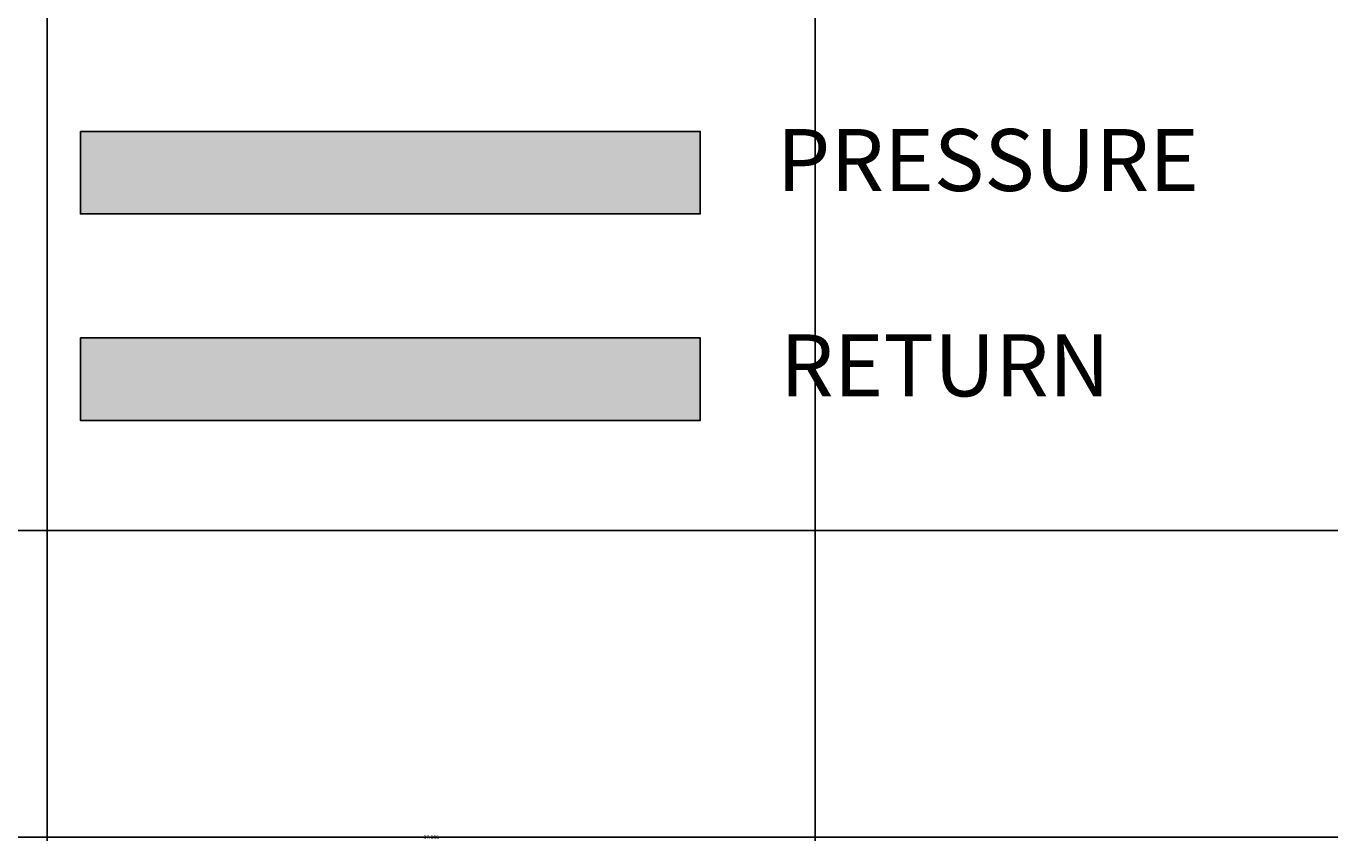
# Model space of a CAD drawing. Units: millimetres. Extents: x -11 to 280, y -4 to 208.
# Tile 2 of 55: x 28 to 91, y -4 to 36. Entities that reach past the tile are written whole.
import ezdxf

# ---------------------------------------------------------------- set-up
doc = ezdxf.new("R2010")
doc.units = ezdxf.units.MM
for name, color, linetype, lineweight in [('M-ANNO-TEXT', 7, 'Continuous', 18), ('M-DIMS', 2, 'Continuous', 18), ('M-HYDR-PRES', 7, 'Continuous', 25), ('M-HYDR-RETN', 7, 'Continuous', 25)]:
    doc.layers.add(name, color=color, linetype=linetype, lineweight=lineweight)
doc.layers.add('M-HYDR-PRES-PATT', color=240, linetype='Continuous', lineweight=13, true_color=0xed1f24)
doc.layers.add('M-HYDR-RETN-PATT', color=114, linetype='Continuous', lineweight=13, true_color=0x139b48)
doc.styles.get("Standard").update_dxf_attribs({"font": 'arial.ttf'})
doc.dimstyles.get("Standard").update_dxf_attribs({"dimtxt": 0.18, "dimasz": 0.18, "dimexe": 0.18, "dimexo": 0.0625, "dimgap": 0.09, "dimtad": 0, "dimtih": 1, "dimtoh": 1, "dimdec": 4, "dimzin": 0, "dimdsep": 46, "dimtxsty": 'Standard', "dimcen": 0.09, "dimadec": 0, "dimazin": 0, "dimtfac": 1, "dimtdec": 4, "dimtofl": 0, "dimtmove": 0, "dimatfit": 3, "dimfxl": 1, "dimtolj": 1, "dimtzin": 0, "dimarcsym": 0})

# ---------------------------------------------------------------- blocks, each defined once
blk = doc.blocks.new('*D4')
at = {"layer": 'Defpoints', "color": 0, "transparency": 16777216}
for p in [(4.763, 84.426), (266.035, 51.733), (266.035, -3.415)]:
    blk.add_point(p, dxfattribs=at)
at = {"layer": 'M-DIMS', "color": 0, "lineweight": -2, "transparency": 16777216}
for p, q in [((4.763, 84.364), (4.763, -3.595)), ((266.035, 51.67), (266.035, -3.595)), ((4.943, -3.415), (134.934, -3.415)), ((265.855, -3.415), (135.864, -3.415))]:
    blk.add_line(p, q, dxfattribs=at)
at = {"layer": 'M-DIMS', "color": 0, "transparency": 16777216}
for points in [[(4.943, -3.385), (4.943, -3.445), (4.763, -3.415)], [(265.855, -3.385), (265.855, -3.445), (266.035, -3.415)]]:
    blk.add_solid(points, dxfattribs=at)
at = {"layer": 'M-DIMS', "color": 0, "transparency": 16777216, "insert": (135.399, -3.415), "char_height": 0.18, "attachment_point": 5}
blk.add_mtext('\\A1;261.27', dxfattribs=at)
blk = doc.blocks.new('*D5')
at = {"layer": 'Defpoints', "color": 0, "transparency": 16777216}
for p in [(24.759, 192.645), (-10.087, 11.435), (261.686, 11.435)]:
    blk.add_point(p, dxfattribs=at)
at = {"layer": 'M-DIMS', "color": 0, "lineweight": -2, "transparency": 16777216}
for p, q in [((24.696, 192.645), (-10.267, 192.645)), ((-10.087, 192.465), (-10.087, 102.222)), ((-10.087, 11.615), (-10.087, 101.858)), ((261.624, 11.435), (-10.267, 11.435))]:
    blk.add_line(p, q, dxfattribs=at)
at = {"layer": 'M-DIMS', "color": 0, "transparency": 16777216}
for points in [[(-10.117, 192.465), (-10.057, 192.465), (-10.087, 192.645)], [(-10.117, 11.615), (-10.057, 11.615), (-10.087, 11.435)]]:
    blk.add_solid(points, dxfattribs=at)
at = {"layer": 'M-DIMS', "color": 0, "transparency": 16777216, "insert": (-10.087, 102.04), "char_height": 0.18, "attachment_point": 5}
blk.add_mtext('\\A1;181.2', dxfattribs=at)
blk = doc.blocks.new('*D23')
at = {"layer": 'Defpoints', "color": 0, "transparency": 16777216}
for p in [(29.201, 153.977), (66.388, 153.977), (66.388, -3.415)]:
    blk.add_point(p, dxfattribs=at)
at = {"layer": 'M-DIMS', "color": 0, "lineweight": -2, "transparency": 16777216}
for p, q in [((29.201, 153.914), (29.201, -3.595)), ((66.388, 153.914), (66.388, -3.595)), ((29.381, -3.415), (47.331, -3.415)), ((66.208, -3.415), (48.258, -3.415))]:
    blk.add_line(p, q, dxfattribs=at)
at = {"layer": 'M-DIMS', "color": 0, "transparency": 16777216}
for points in [[(29.381, -3.385), (29.381, -3.445), (29.201, -3.415)], [(66.208, -3.385), (66.208, -3.445), (66.388, -3.415)]]:
    blk.add_solid(points, dxfattribs=at)
at = {"layer": 'M-DIMS', "color": 0, "transparency": 16777216, "insert": (47.795, -3.415), "char_height": 0.18, "attachment_point": 5}
blk.add_mtext('\\A1;37.186', dxfattribs=at)

msp = doc.modelspace()

# ---------------------------------------------------------------- hatches: boundary and pattern name
at = {"layer": 'M-HYDR-PRES-PATT'}
h = msp.add_hatch(color=256, dxfattribs=at)
h.set_gradient(color1=(237, 31, 36), color2=(237, 31, 36), tint=1)
h.paths.add_polyline_path([(30.8182, 30.7626), (30.8182, 26.7626), (60.8182, 26.7626), (60.8182, 30.7626)])
at = {"layer": 'M-HYDR-RETN-PATT'}
h = msp.add_hatch(color=256, dxfattribs=at)
h.set_gradient(color1=(19, 155, 72), color2=(19, 155, 72), tint=1)
h.paths.add_polyline_path([(60.8182, 16.7626), (60.8182, 20.7626), (30.8182, 20.7626), (30.8182, 16.7626)])

# ---------------------------------------------------------------- linework, layer by layer
at = {"layer": 'M-HYDR-PRES'}
msp.add_lwpolyline([(30.8182, 30.7626), (60.8182, 30.7626), (60.8182, 26.7626), (30.8182, 26.7626)], close=True, dxfattribs=at)
at = {"layer": 'M-HYDR-RETN'}
msp.add_lwpolyline([(30.8182, 20.7626), (60.8182, 20.7626), (60.8182, 16.7626), (30.8182, 16.7626)], close=True, dxfattribs=at)

# ---------------------------------------------------------------- texts
at = {"layer": 'M-ANNO-TEXT', "char_height": 3, "attachment_point": 1}
for s, insert in [('PRESSURE', (64.5255, 30.8753)), ('RETURN', (64.6786, 20.9312))]:
    msp.add_mtext_dynamic_manual_height_columns(s, width=31.695986, gutter_width=12.5, heights=[0], dxfattribs=dict(at, insert=insert))

# ---------------------------------------------------------------- dimensions: what is measured, and where the dimension line sits
at = {"layer": 'M-DIMS'}
dim = msp.add_linear_dim(base=(-10.0865, 11.4346), p1=(24.7588, 192.645), p2=(261.6863, 11.4346), angle=90, dimstyle='Standard', override={"dimdec": 1, "dimlfac": 1, "dimrnd": 0, "dimzin": 0, "dimdsep": 46, "dimlunit": 2}, dxfattribs=at)
dim.commit()
dim.dimension.update_dxf_attribs({"geometry": '*D5', "text_midpoint": (-10.0865, 102.0398)})
for base, p1, p2, override, picture, middle in [((66.3875, -3.4154), (29.2015, 153.9768), (66.3875, 153.9768), {"dimdec": 3, "dimlfac": 1, "dimrnd": 0, "dimzin": 0, "dimdsep": 46, "dimlunit": 2}, '*D23', (47.7945, -3.4154)), ((266.0352, -3.4154), (4.7635, 84.4261), (266.0352, 51.7328), {"dimdec": 2, "dimlfac": 1, "dimrnd": 0, "dimzin": 0, "dimdsep": 46, "dimlunit": 2}, '*D4', (135.3993, -3.4154))]:
    dim = msp.add_linear_dim(base=base, p1=p1, p2=p2, dimstyle='Standard', override=override, dxfattribs=at)
    dim.commit()
    dim.dimension.update_dxf_attribs({"geometry": picture, "text_midpoint": middle})

doc.saveas('drawing.dxf')
